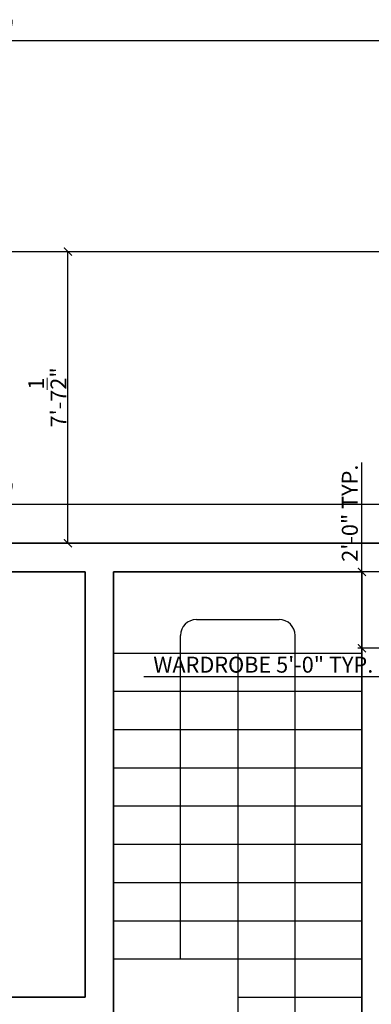
# Model space of a CAD drawing. Units: inches. Extents: x 3283068 to 3284536, y 3240756 to 3241803.
# Tile 16 of 19: x 3283799 to 3283910, y 3241494 to 3241803. Entities that reach past the tile are written whole.
import ezdxf

# ---------------------------------------------------------------- set-up
doc = ezdxf.new("R2010")
doc.units = ezdxf.units.IN
for name, color, linetype, lineweight in [('A-ANNO-DIMS', 2, 'Continuous', 18), ('C-PROP', 7, 'Continuous', 25), ('STAIR', 50, 'Continuous', 25), ('wall', 20, 'Continuous', 35)]:
    doc.layers.add(name, color=color, linetype=linetype, lineweight=lineweight)
doc.styles.get("Standard").update_dxf_attribs({"font": 'arial.ttf'})
doc.dimstyles.new('ISO-25', dxfattribs={"dimtxt": 5, "dimasz": 2.5, "dimexe": 1.25, "dimexo": 0.625, "dimtad": 1, "dimlunit": 4, "dimtxsty": 'Standard', "dimblk": 'ARCHTICK', "dimcen": 2.5, "dimadec": 0, "dimazin": 0, "dimtfac": 1, "dimtmove": 0, "dimatfit": 3, "dimfxl": 1, "dimarcsym": 0})

# ---------------------------------------------------------------- blocks, each defined once
blk = doc.blocks.new('_ArchTick')
at = {"color": 0, "linetype": 'ByBlock', "const_width": 0.15}
blk.add_lwpolyline([(-0.5, -0.5), (0.5, 0.5)], dxfattribs=at)
blk = doc.blocks.new('*D25')
at = {"layer": 'A-ANNO-DIMS', "color": 0, "lineweight": -2, "transparency": 16777216}
for p, q in [((3283339.59, 3241639.73), (3283339.59, 3241652.58)), ((3283339.59, 3241651.33), (3284236.59, 3241651.33)), ((3284236.59, 3241639.73), (3284236.59, 3241652.58))]:
    blk.add_line(p, q, dxfattribs=at)
at = {"layer": 'Defpoints', "color": 0, "transparency": 16777216}
for p in [(3284236.59, 3241651.33), (3283339.59, 3241639.1), (3284236.59, 3241639.1)]:
    blk.add_point(p, dxfattribs=at)
at = {"layer": 'A-ANNO-DIMS', "color": 0, "lineweight": -2, "transparency": 16777216, "xscale": 2.5, "yscale": 2.5, "zscale": 2.5, "rotation": 180}
blk.add_blockref('_ArchTick', (3283339.59, 3241651.33), dxfattribs=at)
at = {"layer": 'A-ANNO-DIMS', "color": 0, "lineweight": -2, "transparency": 16777216, "xscale": 2.5, "yscale": 2.5, "zscale": 2.5}
blk.add_blockref('_ArchTick', (3284236.59, 3241651.33), dxfattribs=at)
at = {"layer": 'A-ANNO-DIMS', "color": 0, "transparency": 16777216, "insert": (3283788.09, 3241654.51), "char_height": 5, "attachment_point": 5}
blk.add_mtext('74\'-9"', dxfattribs=at)
blk = doc.blocks.new('*D34')
at = {"layer": 'A-ANNO-DIMS', "color": 0, "lineweight": -2, "transparency": 16777216}
for p, q in [((3283800.58, 3241730.6), (3283815.48, 3241730.6)), ((3283814.23, 3241639.1), (3283814.23, 3241730.6)), ((3283800.58, 3241639.1), (3283815.48, 3241639.1))]:
    blk.add_line(p, q, dxfattribs=at)
at = {"layer": 'Defpoints', "color": 0, "transparency": 16777216}
for p in [(3283799.96, 3241730.6), (3283814.23, 3241730.6), (3283799.96, 3241639.1)]:
    blk.add_point(p, dxfattribs=at)
at = {"layer": 'A-ANNO-DIMS', "color": 0, "lineweight": -2, "transparency": 16777216, "xscale": 2.5, "yscale": 2.5, "zscale": 2.5}
for p, rotation in [((3283814.23, 3241730.6), 90), ((3283814.23, 3241639.1), 270)]:
    blk.add_blockref('_ArchTick', p, dxfattribs=dict(at, rotation=rotation))
at = {"layer": 'A-ANNO-DIMS', "color": 0, "transparency": 16777216, "insert": (3283807.75, 3241684.85), "char_height": 5, "attachment_point": 5, "rotation": 90}
blk.add_mtext('7\'-7{\\H1x;\\S1/2;}"', dxfattribs=at)
blk = doc.blocks.new('*D49')
at = {"layer": 'A-ANNO-DIMS', "color": 0, "lineweight": -2, "transparency": 16777216}
for p, q in [((3283915.59, 3241605.48), (3283915.59, 3241595.85)), ((3283975.59, 3241605.48), (3283975.59, 3241595.85)), ((3283915.59, 3241597.1), (3283838.08, 3241597.1)), ((3283975.59, 3241597.1), (3283915.59, 3241597.1))]:
    blk.add_line(p, q, dxfattribs=at)
at = {"layer": 'Defpoints', "color": 0, "transparency": 16777216}
for p in [(3283915.59, 3241606.1), (3283975.59, 3241606.1), (3283915.59, 3241597.1)]:
    blk.add_point(p, dxfattribs=at)
at = {"layer": 'A-ANNO-DIMS', "color": 0, "lineweight": -2, "transparency": 16777216, "xscale": 2.5, "yscale": 2.5, "zscale": 2.5}
for p, rotation in [((3283915.59, 3241597.1), 180.0000000004447), ((3283975.59, 3241597.1), 4.446843e-10)]:
    blk.add_blockref('_ArchTick', p, dxfattribs=dict(at, rotation=rotation))
at = {"layer": 'A-ANNO-DIMS', "color": 0, "transparency": 16777216, "insert": (3283875.59, 3241600.31), "char_height": 5, "attachment_point": 5}
blk.add_mtext('WARDROBE 5\'-0" TYP.', dxfattribs=at)
blk = doc.blocks.new('*D50')
at = {"layer": 'A-ANNO-DIMS', "color": 0, "lineweight": -2, "transparency": 16777216}
for p, q in [((3283906.59, 3241630.1), (3283906.59, 3241664.42)), ((3283914.96, 3241630.1), (3283905.34, 3241630.1)), ((3283906.59, 3241606.1), (3283906.59, 3241630.1)), ((3283914.96, 3241606.1), (3283905.34, 3241606.1))]:
    blk.add_line(p, q, dxfattribs=at)
at = {"layer": 'Defpoints', "color": 0, "transparency": 16777216}
for p in [(3283906.59, 3241630.1), (3283915.59, 3241630.1), (3283915.59, 3241606.1)]:
    blk.add_point(p, dxfattribs=at)
at = {"layer": 'A-ANNO-DIMS', "color": 0, "lineweight": -2, "transparency": 16777216, "xscale": 2.5, "yscale": 2.5, "zscale": 2.5}
for p, rotation in [((3283906.59, 3241630.1), 90), ((3283906.59, 3241606.1), 270)]:
    blk.add_blockref('_ArchTick', p, dxfattribs=dict(at, rotation=rotation))
at = {"layer": 'A-ANNO-DIMS', "color": 0, "transparency": 16777216, "insert": (3283903.41, 3241648.51), "char_height": 5, "attachment_point": 5, "rotation": 90}
blk.add_mtext('2\'-0" TYP.', dxfattribs=at)
blk = doc.blocks.new('*D63')
at = {"layer": 'A-ANNO-DIMS', "color": 0, "lineweight": -2, "transparency": 16777216}
for p, q in [((3283248.09, 3241083.23), (3283248.09, 3241798.08)), ((3283248.09, 3241796.83), (3284328.09, 3241796.83)), ((3284328.09, 3241083.23), (3284328.09, 3241798.08))]:
    blk.add_line(p, q, dxfattribs=at)
at = {"layer": 'Defpoints', "color": 0, "transparency": 16777216}
for p in [(3284328.09, 3241796.83), (3283248.09, 3241082.6), (3284328.09, 3241082.6)]:
    blk.add_point(p, dxfattribs=at)
at = {"layer": 'A-ANNO-DIMS', "color": 0, "lineweight": -2, "transparency": 16777216, "xscale": 2.5, "yscale": 2.5, "zscale": 2.5, "rotation": 180}
blk.add_blockref('_ArchTick', (3283248.09, 3241796.83), dxfattribs=at)
at = {"layer": 'A-ANNO-DIMS', "color": 0, "lineweight": -2, "transparency": 16777216, "xscale": 2.5, "yscale": 2.5, "zscale": 2.5}
blk.add_blockref('_ArchTick', (3284328.09, 3241796.83), dxfattribs=at)
at = {"layer": 'A-ANNO-DIMS', "color": 0, "transparency": 16777216, "insert": (3283788.09, 3241800.01), "char_height": 5, "attachment_point": 5}
blk.add_mtext('90\'-0"', dxfattribs=at)

msp = doc.modelspace()

# ---------------------------------------------------------------- linework, layer by layer
at = {"layer": 'C-PROP'}
msp.add_line((3283248.089, 3241730.602), (3284328.089, 3241730.602), dxfattribs=at)
at = {"layer": 'STAIR'}
for p, q in [((3283854.619, 3241615.107), (3283880.56, 3241615.107)), ((3283849.619, 3241508.602), (3283849.619, 3241610.107)), ((3283885.56, 3241484.602), (3283885.56, 3241610.107)), ((3283828.589, 3241604.602), (3283906.589, 3241604.602)), ((3283867.589, 3241604.602), (3283867.589, 3241460.602)), ((3283828.589, 3241592.602), (3283906.589, 3241592.602)), ((3283828.589, 3241580.602), (3283906.589, 3241580.602)), ((3283828.589, 3241568.602), (3283906.589, 3241568.602)), ((3283828.589, 3241556.602), (3283906.589, 3241556.602)), ((3283828.589, 3241544.602), (3283906.589, 3241544.602)), ((3283828.589, 3241532.602), (3283906.589, 3241532.602)), ((3283828.589, 3241520.602), (3283906.589, 3241520.602)), ((3283828.589, 3241508.602), (3283906.589, 3241508.602)), ((3283867.589, 3241496.602), (3283906.589, 3241496.602))]:
    msp.add_line(p, q, dxfattribs=at)
for centre, start, end in [((3283854.619, 3241610.107), 90, 180), ((3283880.56, 3241610.107), 0, 90)]:
    msp.add_arc(centre, 5, start, end, dxfattribs=at)
at = {"layer": 'wall'}
for p, q in [((3283339.589, 3241639.102), (3284236.589, 3241639.102)), ((3283665.089, 3241630.102), (3283819.589, 3241630.102)), ((3283819.589, 3241630.102), (3283819.589, 3241496.602)), ((3283828.589, 3241630.102), (3283828.589, 3241328.853)), ((3283828.589, 3241630.102), (3283906.589, 3241630.102)), ((3283906.589, 3241630.102), (3283906.589, 3241198.102)), ((3283665.089, 3241496.602), (3283819.589, 3241496.602))]:
    msp.add_line(p, q, dxfattribs=at)

# ---------------------------------------------------------------- dimensions: what is measured, and where the dimension line sits
at = {"layer": 'A-ANNO-DIMS'}
for base, p1, p2, override, picture, middle in [((3284328.089, 3241796.827), (3283248.089, 3241082.602), (3284328.089, 3241082.602), {"dimdec": 1, "dimlfac": 1, "dimrnd": 0, "dimzin": 1, "dimdsep": 46, "dimlunit": 4, "dimfrac": 2}, '*D63', (3283788.089, 3241800.005)), ((3284236.589, 3241651.334), (3283339.589, 3241639.102), (3284236.589, 3241639.102), {"dimclrd": 0, "dimclre": 0, "dimclrt": 0}, '*D25', (3283788.089, 3241654.512))]:
    dim = msp.add_linear_dim(base=base, p1=p1, p2=p2, dimstyle='ISO-25', override=override, dxfattribs=at)
    dim.commit()
    dim.dimension.update_dxf_attribs({"geometry": picture, "text_midpoint": middle})
dim = msp.add_linear_dim(base=(3283814.226, 3241730.602), p1=(3283799.957, 3241639.102), p2=(3283799.957, 3241730.602), angle=90, dimstyle='ISO-25', override={"dimclrd": 0, "dimclre": 0, "dimclrt": 0}, dxfattribs=at)
dim.commit()
dim.dimension.update_dxf_attribs({"geometry": '*D34', "text_midpoint": (3283807.747, 3241684.852)})
for base, p1, p2, angle, text, picture, middle in [((3283906.589, 3241630.102), (3283915.589, 3241606.102), (3283915.589, 3241630.102), 90, '<> TYP.', '*D50', (3283903.412, 3241648.509)), ((3283915.589, 3241597.102), (3283975.589, 3241606.102), (3283915.589, 3241606.102), 180, 'WARDROBE <> TYP.', '*D49', (3283875.585, 3241600.314))]:
    dim = msp.add_linear_dim(base=base, p1=p1, p2=p2, angle=angle, text=text, dimstyle='ISO-25', override={"dimdec": 1, "dimlfac": 1, "dimrnd": 0, "dimzin": 1, "dimdsep": 46, "dimlunit": 4, "dimfrac": 2}, dxfattribs=at)
    dim.commit()
    dim.dimension.update_dxf_attribs({"geometry": picture, "text_midpoint": middle})

doc.saveas('drawing.dxf')
